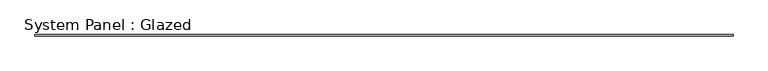
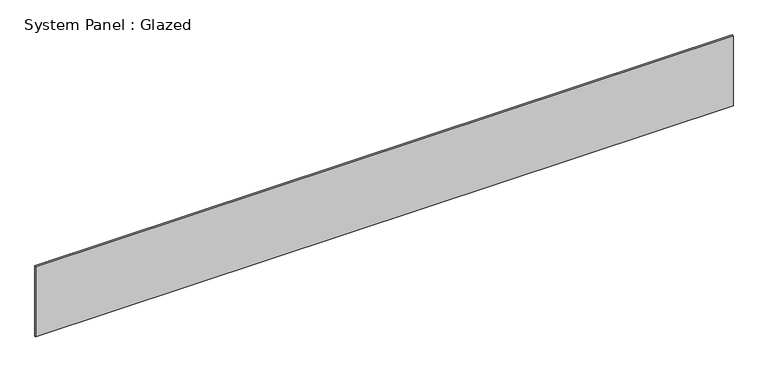
"""IFC4 building model written with IfcOpenShell, lengths in millimetres: plate geometry, System Panel : Glazed."""

from ifc_helpers import new_model, si_unit, origin, origin_with_axes, place, context, project, spatial, polyline, outline, extrude, source, transform, mapped, element, save


def system_panel_glazed_e5b44d49(model_context):
    return source(origin(), model_context, "Body", "SweptSolid", [
        extrude(outline(polyline([(6852.8114633, 19.05), (-6852.8114633, 19.05), (-6852.8114633, 44.45), (6852.8114633, 44.45), (6852.8114633, 19.05)])), origin_with_axes(), (0.0, 0.0, 1.0), 1460.5),
    ])


if __name__ == "__main__":
    model = new_model("IFC4")
    model_context = context("Model", 3, world=origin())
    ifc_project = project(units=[si_unit("LENGTHUNIT", "METRE", prefix="MILLI")], contexts=[model_context])
    site = spatial("IfcSite", under=ifc_project)
    building = spatial("IfcBuilding", under=site)
    placement = place(None, origin())
    system_panel_glazed_shape = system_panel_glazed_e5b44d49(model_context)
    element("IfcPlate", 1, ObjectType="System Panel : Glazed", at=placement, inside=building, context=model_context, shape_type="MappedRepresentation", body=[
        mapped(system_panel_glazed_shape, transform((0.0, 0.0, 0.0), x_axis=(1.0, 0.0, 0.0), y_axis=(0.0, 1.0, 0.0), z_axis=(0.0, 0.0, 1.0))),
    ])
    save(model, "model.ifc")

# Revit data of these elements
# Type "System Panel : Glazed"
#   Construction Type Id = "GSP4R"
#   Analytic Construction = "1/8 in Pilkington single glazing"
#   Visual Light Transmittance = 0.9
#   Solar Heat Gain Coefficient = 0.86
#   Heat Transfer Coefficient (U) = 1.18115 BTU/(h·ft²·°F)
# Element 1 (IfcPlate, "System Panel : Glazed")
#   Materials on its faces: "Glass"
# Materials
#   "Glass": class "Glass", colour RGB 0 128 192, transparency 0.75, Description = "Soda Lime Glass", Cost = 0
